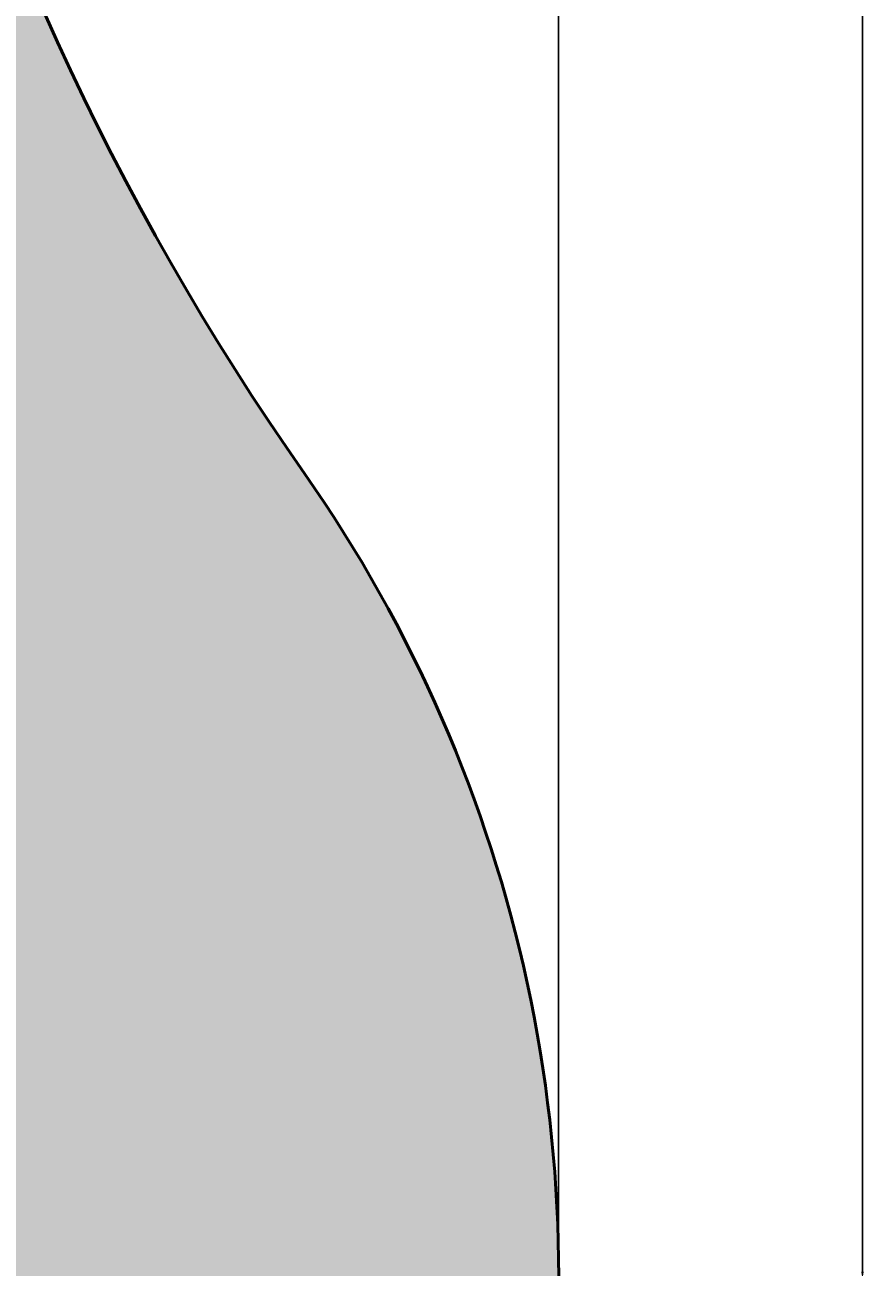
# Model space of a CAD drawing. Units: inches. Extents: x -13 to 107, y -48 to 102.
# Tile 9 of 13: x 48 to 68, y 14 to 43. Entities that reach past the tile are written whole.
import ezdxf

# ---------------------------------------------------------------- set-up
doc = ezdxf.new("R2010")
doc.units = ezdxf.units.IN
doc.header["$MEASUREMENT"] = 0
for name, color, linetype, lineweight in [('M-DIMS', 2, 'Continuous', 18), ('M-HATC', 8, 'Continuous', 18), ('M-OUTL', 7, 'Continuous', 50)]:
    doc.layers.add(name, color=color, linetype=linetype, lineweight=lineweight)
doc.styles.get("Standard").update_dxf_attribs({"font": 'arial.ttf'})
doc.dimstyles.get("Standard").update_dxf_attribs({"dimtxt": 0.18, "dimasz": 0.18, "dimexe": 0.18, "dimexo": 0.0625, "dimgap": 0.09, "dimtad": 0, "dimtih": 1, "dimtoh": 1, "dimdec": 4, "dimzin": 0, "dimdsep": 46, "dimtxsty": 'Standard', "dimcen": 0.09, "dimadec": 0, "dimazin": 0, "dimtfac": 1, "dimtdec": 4, "dimtofl": 0, "dimtmove": 0, "dimatfit": 3, "dimfxl": 1, "dimtolj": 1, "dimtzin": 0, "dimarcsym": 0})

# ---------------------------------------------------------------- blocks, each defined once
blk = doc.blocks.new('*D1')
at = {"layer": 'Defpoints', "color": 0, "transparency": 16777216}
for p in [(60.544, 101.543), (-5.45, 13.883), (60.544, 13.883)]:
    blk.add_point(p, dxfattribs=at)
at = {"layer": 'M-DIMS', "color": 0, "lineweight": -2, "transparency": 16777216}
for p, q in [((-5.45, 13.945), (-5.45, 101.723)), ((60.544, 13.945), (60.544, 101.723)), ((-5.27, 101.543), (27.328, 101.543)), ((60.364, 101.543), (27.766, 101.543))]:
    blk.add_line(p, q, dxfattribs=at)
at = {"layer": 'M-DIMS', "color": 0, "transparency": 16777216}
for points in [[(-5.27, 101.573), (-5.27, 101.513), (-5.45, 101.543)], [(60.364, 101.573), (60.364, 101.513), (60.544, 101.543)]]:
    blk.add_solid(points, dxfattribs=at)
at = {"layer": 'M-DIMS', "color": 0, "transparency": 16777216, "insert": (27.547, 101.543), "char_height": 0.18, "attachment_point": 5}
blk.add_mtext('\\A1;66', dxfattribs=at)
blk = doc.blocks.new('*D4')
at = {"layer": 'Defpoints', "color": 0, "transparency": 16777216}
for p in [(27.547, 78.408), (67.679, 78.408), (27.547, 13.408)]:
    blk.add_point(p, dxfattribs=at)
at = {"layer": 'M-DIMS', "color": 0, "lineweight": -2, "transparency": 16777216}
for p, q in [((27.609, 78.408), (67.859, 78.408)), ((67.679, 78.228), (67.679, 46.09)), ((67.679, 13.588), (67.679, 45.726)), ((27.609, 13.408), (67.859, 13.408))]:
    blk.add_line(p, q, dxfattribs=at)
at = {"layer": 'M-DIMS', "color": 0, "transparency": 16777216}
for points in [[(67.649, 78.228), (67.709, 78.228), (67.679, 78.408)], [(67.649, 13.588), (67.709, 13.588), (67.679, 13.408)]]:
    blk.add_solid(points, dxfattribs=at)
at = {"layer": 'M-DIMS', "color": 0, "transparency": 16777216, "insert": (67.679, 45.908), "char_height": 0.18, "attachment_point": 5}
blk.add_mtext('\\A1;65', dxfattribs=at)

msp = doc.modelspace()

# ---------------------------------------------------------------- hatches: boundary and pattern name
at = {"layer": 'M-HATC'}
h = msp.add_hatch(color=256, dxfattribs=at)
h.set_gradient(color1=(88, 186, 72), color2=(241, 235, 31), tint=1)
h.paths.add_polyline_path([(45.86, -14.044, 0.420873), (54.577, 32.339, -0.184081), (43.437, 76.537, 1.124637), (11.657, 76.537, -0.184081), (0.517, 32.339, 0.420873), (9.234, -14.044, -0.304084), (17.743, -34.622, 1.220926), (37.351, -34.622, -0.304084)])
h.paths.add_polyline_path([(33.479, -5.692, 0.859727), (21.615, -5.692, -0.111692), (13.972, -1.28, 0.859727), (8.04, 8.995, -0.111692), (8.04, 17.82, 0.859727), (13.972, 28.095, -0.111692), (21.615, 32.508, 0.859727), (33.479, 32.508, -0.111692), (41.122, 28.095, 0.859727), (47.054, 17.82, -0.111692), (47.054, 8.995, 0.859727), (41.122, -1.28, -0.111692)], flags=16)
h.paths.add_polyline_path([(32.547, -36.592, -1), (22.547, -36.592, -1)], flags=16)
h.paths.add_polyline_path([(17.547, 78.408, -1), (37.547, 78.408, -1)], flags=16)

# ---------------------------------------------------------------- linework, layer by layer
at = {"layer": 'M-OUTL'}
for centre, radius, start, end in [((106.998, 69.054), 64, 173.28544, 215.00666), ((27.547, 13.408), 33, 303.707, 35.0067)]:
    msp.add_arc(centre, radius, start, end, dxfattribs=at)

# ---------------------------------------------------------------- dimensions: what is measured, and where the dimension line sits
at = {"layer": 'M-DIMS'}
dim = msp.add_linear_dim(base=(60.544, 101.543), p1=(-5.45, 13.883), p2=(60.544, 13.883), dimstyle='Standard', override={"dimdec": 0, "dimlfac": 1, "dimrnd": 0, "dimzin": 0, "dimdsep": 46, "dimlunit": 2}, dxfattribs=at)
dim.commit()
dim.dimension.update_dxf_attribs({"geometry": '*D1', "text_midpoint": (27.547, 101.543)})
dim = msp.add_linear_dim(base=(67.679, 78.408), p1=(27.547, 13.408), p2=(27.547, 78.408), angle=90, dimstyle='Standard', override={"dimdec": 0, "dimlfac": 1, "dimrnd": 0, "dimzin": 0, "dimdsep": 46, "dimlunit": 2}, dxfattribs=at)
dim.commit()
dim.dimension.update_dxf_attribs({"geometry": '*D4', "text_midpoint": (67.679, 45.908)})

doc.saveas('drawing.dxf')
